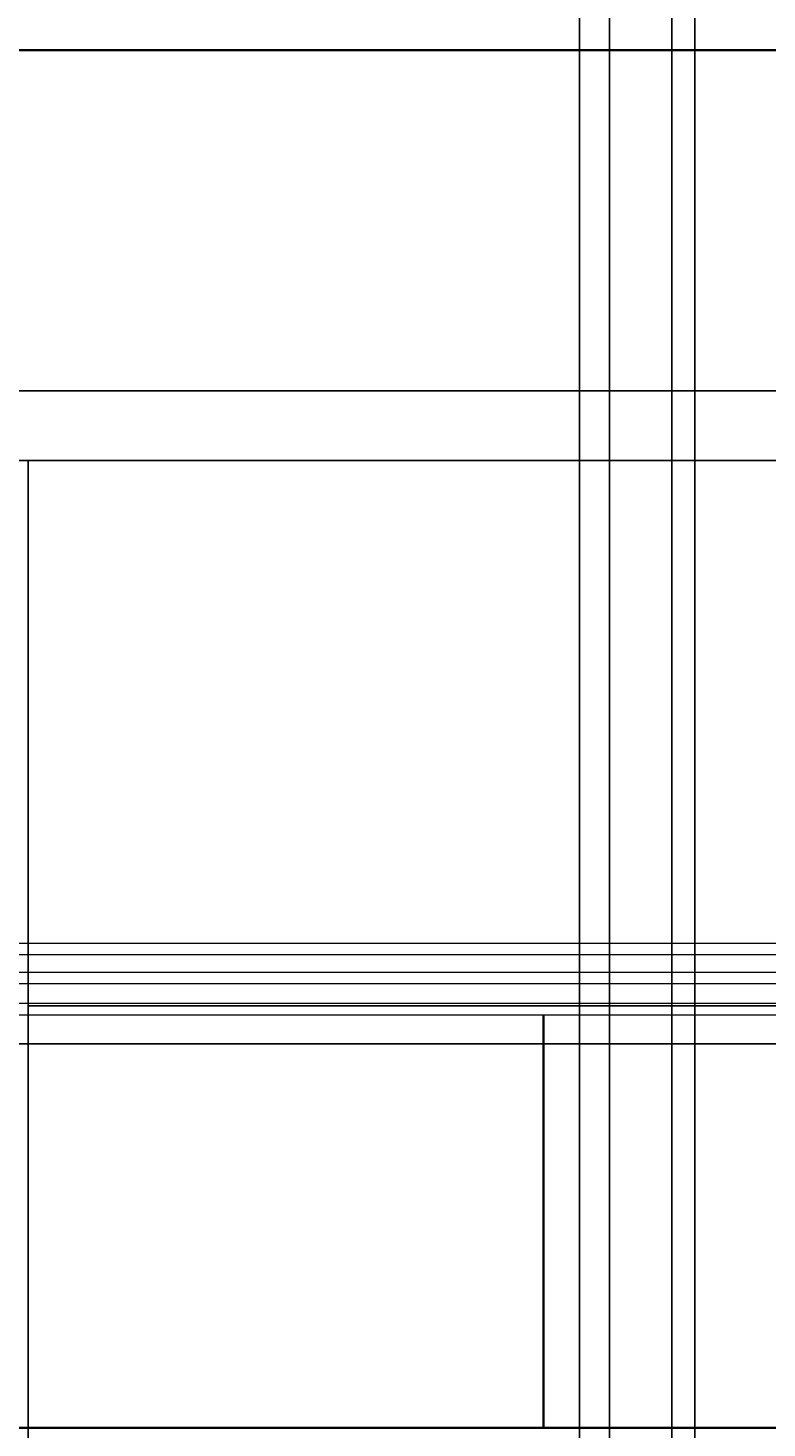
# Model space of a CAD drawing. Units: inches. Extents: x -13 to 809, y 112 to 656.
# Tile 16 of 55: x 210 to 274, y 325 to 446. Entities that reach past the tile are written whole.
import ezdxf

# ---------------------------------------------------------------- set-up
doc = ezdxf.new("R2010")
doc.units = ezdxf.units.IN
doc.header["$MEASUREMENT"] = 0
for name, color, linetype, lineweight in [('A-ANNO-DIMS', 2, 'Continuous', 18), ('A-ELEV', 7, 'Continuous', 35), ('A-ELEV-PATT', 8, 'Continuous', 13), ('A-GLAZ', 4, 'Continuous', 25)]:
    doc.layers.add(name, color=color, linetype=linetype, lineweight=lineweight)
doc.styles.get("Standard").update_dxf_attribs({"font": 'arial.ttf'})
doc.dimstyles.get("Standard").update_dxf_attribs({"dimtxt": 0.625, "dimasz": 0.18, "dimexe": 0.18, "dimexo": 0.0625, "dimgap": 0.09, "dimtad": 0, "dimtih": 1, "dimtoh": 1, "dimdec": 4, "dimzin": 0, "dimdsep": 46, "dimlunit": 4, "dimtxsty": 'Standard', "dimcen": 0.09, "dimadec": 0, "dimazin": 0, "dimtfac": 1, "dimtdec": 4, "dimtofl": 0, "dimtmove": 0, "dimatfit": 3, "dimfxl": 1, "dimtolj": 1, "dimtzin": 0, "dimarcsym": 0})

# ---------------------------------------------------------------- blocks, each defined once
blk = doc.blocks.new('*D39')
at = {"layer": 'A-ANNO-DIMS', "color": 0, "lineweight": -2, "transparency": 16777216}
for p, q in [((341.34, 524.28), (-12.1, 524.28)), ((-11.92, 524.1), (-11.92, 406.78)), ((-11.92, 288.63), (-11.92, 405.96)), ((341.34, 288.45), (-12.1, 288.45))]:
    blk.add_line(p, q, dxfattribs=at)
at = {"layer": 'A-ANNO-DIMS', "color": 0, "transparency": 16777216}
for points in [[(-11.95, 524.1), (-11.89, 524.1), (-11.92, 524.28)], [(-11.95, 288.63), (-11.89, 288.63), (-11.92, 288.45)]]:
    blk.add_solid(points, dxfattribs=at)
at = {"layer": 'Defpoints', "color": 0, "transparency": 16777216}
for p in [(-11.92, 524.28), (341.41, 524.28), (341.41, 288.45)]:
    blk.add_point(p, dxfattribs=at)
at = {"layer": 'A-ANNO-DIMS', "color": 0, "transparency": 16777216, "insert": (-11.92, 406.37), "char_height": 0.625, "attachment_point": 5}
blk.add_mtext('\\A1;235.83', dxfattribs=at)
blk = doc.blocks.new('*D41')
at = {"layer": 'A-ANNO-DIMS', "color": 0, "lineweight": -2, "transparency": 16777216}
for p, q in [((471.04, 357.98), (-12.1, 357.98)), ((-11.92, 357.8), (-11.92, 335.98)), ((-11.92, 313.35), (-11.92, 335.16)), ((471.04, 313.17), (-12.1, 313.17))]:
    blk.add_line(p, q, dxfattribs=at)
at = {"layer": 'A-ANNO-DIMS', "color": 0, "transparency": 16777216}
for points in [[(-11.95, 357.8), (-11.89, 357.8), (-11.92, 357.98)], [(-11.95, 313.35), (-11.89, 313.35), (-11.92, 313.17)]]:
    blk.add_solid(points, dxfattribs=at)
at = {"layer": 'Defpoints', "color": 0, "transparency": 16777216}
for p in [(-11.92, 357.98), (471.1, 357.98), (471.1, 313.17)]:
    blk.add_point(p, dxfattribs=at)
at = {"layer": 'A-ANNO-DIMS', "color": 0, "transparency": 16777216, "insert": (-11.92, 335.57), "char_height": 0.625, "attachment_point": 5}
blk.add_mtext('\\A1;44.81', dxfattribs=at)
blk = doc.blocks.new('*D42')
at = {"layer": 'A-ANNO-DIMS', "color": 0, "lineweight": -2, "transparency": 16777216}
for p, q in [((471.04, 414.86), (-12.1, 414.86)), ((-11.92, 414.68), (-11.92, 386.83)), ((-11.92, 358.16), (-11.92, 386.01)), ((471.04, 357.98), (-12.1, 357.98))]:
    blk.add_line(p, q, dxfattribs=at)
at = {"layer": 'A-ANNO-DIMS', "color": 0, "transparency": 16777216}
for points in [[(-11.95, 414.68), (-11.89, 414.68), (-11.92, 414.86)], [(-11.95, 358.16), (-11.89, 358.16), (-11.92, 357.98)]]:
    blk.add_solid(points, dxfattribs=at)
at = {"layer": 'Defpoints', "color": 0, "transparency": 16777216}
for p in [(-11.92, 414.86), (471.1, 414.86), (471.1, 357.98)]:
    blk.add_point(p, dxfattribs=at)
at = {"layer": 'A-ANNO-DIMS', "color": 0, "transparency": 16777216, "insert": (-11.92, 386.42), "char_height": 0.625, "attachment_point": 5}
blk.add_mtext('\\A1;56.88', dxfattribs=at)
blk = doc.blocks.new('*D43')
at = {"layer": 'A-ANNO-DIMS', "color": 0, "lineweight": -2, "transparency": 16777216}
for p, q in [((471.04, 470.88), (-12.1, 470.88)), ((-11.92, 470.7), (-11.92, 443.28)), ((-11.92, 415.04), (-11.92, 442.46)), ((471.04, 414.86), (-12.1, 414.86))]:
    blk.add_line(p, q, dxfattribs=at)
at = {"layer": 'A-ANNO-DIMS', "color": 0, "transparency": 16777216}
for points in [[(-11.95, 470.7), (-11.89, 470.7), (-11.92, 470.88)], [(-11.95, 415.04), (-11.89, 415.04), (-11.92, 414.86)]]:
    blk.add_solid(points, dxfattribs=at)
at = {"layer": 'Defpoints', "color": 0, "transparency": 16777216}
for p in [(-11.92, 470.88), (471.1, 470.88), (471.1, 414.86)]:
    blk.add_point(p, dxfattribs=at)
at = {"layer": 'A-ANNO-DIMS', "color": 0, "transparency": 16777216, "insert": (-11.92, 442.87), "char_height": 0.625, "attachment_point": 5}
blk.add_mtext('\\A1;56.02', dxfattribs=at)
blk = doc.blocks.new('*D46')
at = {"layer": 'A-ANNO-DIMS', "color": 0, "lineweight": -2, "transparency": 16777216}
for p, q in [((160.98, 408.79), (807.77, 408.79)), ((807.59, 408.61), (807.59, 367.07)), ((807.59, 324.7), (807.59, 366.25)), ((160.98, 324.52), (807.77, 324.52))]:
    blk.add_line(p, q, dxfattribs=at)
at = {"layer": 'A-ANNO-DIMS', "color": 0, "transparency": 16777216}
for points in [[(807.56, 408.61), (807.62, 408.61), (807.59, 408.79)], [(807.56, 324.7), (807.62, 324.7), (807.59, 324.52)]]:
    blk.add_solid(points, dxfattribs=at)
at = {"layer": 'Defpoints', "color": 0, "transparency": 16777216}
for p in [(160.92, 408.79), (807.59, 408.79), (160.92, 324.52)]:
    blk.add_point(p, dxfattribs=at)
at = {"layer": 'A-ANNO-DIMS', "color": 0, "transparency": 16777216, "insert": (807.59, 366.66), "char_height": 0.625, "attachment_point": 5}
blk.add_mtext('\\A1;84.27', dxfattribs=at)
blk = doc.blocks.new('*D112')
at = {"layer": 'A-ANNO-DIMS', "color": 0, "lineweight": -2, "transparency": 16777216}
for p, q in [((210.08, 361.23), (210.08, 112.34)), ((275.71, 361.23), (275.71, 112.34)), ((210.26, 112.52), (241.75, 112.52)), ((275.53, 112.52), (244.04, 112.52))]:
    blk.add_line(p, q, dxfattribs=at)
at = {"layer": 'A-ANNO-DIMS', "color": 0, "transparency": 16777216}
for points in [[(210.26, 112.55), (210.26, 112.49), (210.08, 112.52)], [(275.53, 112.55), (275.53, 112.49), (275.71, 112.52)]]:
    blk.add_solid(points, dxfattribs=at)
at = {"layer": 'Defpoints', "color": 0, "transparency": 16777216}
for p in [(210.08, 361.29), (275.71, 361.29), (275.71, 112.52)]:
    blk.add_point(p, dxfattribs=at)
at = {"layer": 'A-ANNO-DIMS', "color": 0, "transparency": 16777216, "insert": (242.9, 112.52), "char_height": 0.625, "attachment_point": 5}
blk.add_mtext('\\A1;65.64', dxfattribs=at)
blk = doc.blocks.new('*D116')
at = {"layer": 'A-ANNO-DIMS', "color": 0, "lineweight": -2, "transparency": 16777216}
for p, q in [((258.1, 210.85), (258.1, 655.96)), ((258.28, 655.78), (258.5, 655.78)), ((260.52, 655.78), (260.31, 655.78)), ((260.7, 207.43), (260.7, 655.96))]:
    blk.add_line(p, q, dxfattribs=at)
at = {"layer": 'A-ANNO-DIMS', "color": 0, "transparency": 16777216}
for points in [[(258.28, 655.81), (258.28, 655.75), (258.1, 655.78)], [(260.52, 655.81), (260.52, 655.75), (260.7, 655.78)]]:
    blk.add_solid(points, dxfattribs=at)
at = {"layer": 'Defpoints', "color": 0, "transparency": 16777216}
for p in [(260.7, 655.78), (258.1, 210.78), (260.7, 207.37)]:
    blk.add_point(p, dxfattribs=at)
at = {"layer": 'A-ANNO-DIMS', "color": 0, "transparency": 16777216, "insert": (259.4, 655.78), "char_height": 0.625, "attachment_point": 5}
blk.add_mtext('\\A1;2.60', dxfattribs=at)
blk = doc.blocks.new('*D119')
at = {"layer": 'A-ANNO-DIMS', "color": 0, "lineweight": -2, "transparency": 16777216}
for p, q in [((265.9486, 655.782835), (265.7686, 655.782835)), ((266.1286, 207.43492), (266.1286, 655.962835)), ((268.1286, 207.43492), (268.1286, 655.962835)), ((268.3086, 655.782835), (268.4886, 655.782835))]:
    blk.add_line(p, q, dxfattribs=at)
at = {"layer": 'A-ANNO-DIMS', "color": 0, "transparency": 16777216}
for points in [[(265.9486, 655.812835), (265.9486, 655.752835), (266.1286, 655.782835)], [(268.3086, 655.812835), (268.3086, 655.752835), (268.1286, 655.782835)]]:
    blk.add_solid(points, dxfattribs=at)
at = {"layer": 'Defpoints', "color": 0, "transparency": 16777216}
for p in [(268.1286, 655.782835), (266.1286, 207.37242), (268.1286, 207.37242)]:
    blk.add_point(p, dxfattribs=at)
at = {"layer": 'A-ANNO-DIMS', "color": 0, "transparency": 16777216, "insert": (267.1286, 655.782835), "char_height": 0.625, "attachment_point": 5}
blk.add_mtext('\\A1;2.00', dxfattribs=at)

msp = doc.modelspace()

# ---------------------------------------------------------------- linework, layer by layer
at = {"layer": 'A-ELEV'}
for p, q in [((113.0469, 444.5199), (319.5074, 444.5199)), ((254.968, 360.5199), (254.968, 324.5199)), ((113.0469, 324.5199), (319.5074, 324.5199))]:
    msp.add_line(p, q, dxfattribs=at)
at = {"layer": 'A-ELEV-PATT'}
for p, q in [((113.0469, 366.753), (319.5074, 366.753)), ((113.0469, 365.753), (319.5074, 365.753)), ((113.0469, 364.2343), (319.5074, 364.2343)), ((113.0469, 363.2343), (319.5074, 363.2343)), ((113.0469, 361.5199), (319.5074, 361.5199)), ((113.0469, 360.5199), (319.5074, 360.5199))]:
    msp.add_line(p, q, dxfattribs=at)
at = {"layer": 'A-GLAZ'}
msp.add_lwpolyline([(210.0791, 408.7939), (275.7145, 408.7939), (275.7145, 361.2915), (210.0791, 361.2915)], close=True, dxfattribs=at)

# ---------------------------------------------------------------- dimensions: what is measured, and where the dimension line sits
at = {"layer": 'A-ANNO-DIMS'}
for base, p1, p2, picture, middle in [((260.7048, 655.7828), (258.1022, 210.7849), (260.7048, 207.3724), '*D116', (259.4035, 655.7828)), ((268.1286, 655.7828), (266.1286, 207.3724), (268.1286, 207.3724), '*D119', (267.1286, 655.7828)), ((275.7145, 112.5199), (210.0791, 361.2915), (275.7145, 361.2915), '*D112', (242.8968, 112.5199))]:
    dim = msp.add_linear_dim(base=base, p1=p1, p2=p2, dimstyle='Standard', override={"dimdec": 2, "dimlfac": 1, "dimrnd": 0, "dimzin": 0, "dimdsep": 46, "dimlunit": 2}, dxfattribs=at)
    dim.commit()
    dim.dimension.update_dxf_attribs({"geometry": picture, "text_midpoint": middle})
for base, p1, p2, picture, middle in [((-11.9191, 524.281), (341.4072, 288.4508), (341.4072, 524.281), '*D39', (-11.9191, 406.3659)), ((-11.9191, 470.8765), (471.0998, 414.8594), (471.0998, 470.8765), '*D43', (-11.9191, 442.8679)), ((-11.9191, 414.8594), (471.0998, 357.9804), (471.0998, 414.8594), '*D42', (-11.9191, 386.4199)), ((807.5888, 408.7939), (160.9184, 324.5199), (160.9184, 408.7939), '*D46', (807.5888, 366.6569)), ((-11.9191, 357.9804), (471.0998, 313.1667), (471.0998, 357.9804), '*D41', (-11.9191, 335.5735))]:
    dim = msp.add_linear_dim(base=base, p1=p1, p2=p2, angle=90, dimstyle='Standard', override={"dimdec": 2, "dimlfac": 1, "dimrnd": 0, "dimzin": 0, "dimdsep": 46, "dimlunit": 2}, dxfattribs=at)
    dim.commit()
    dim.dimension.update_dxf_attribs({"geometry": picture, "text_midpoint": middle})

doc.saveas('drawing.dxf')
